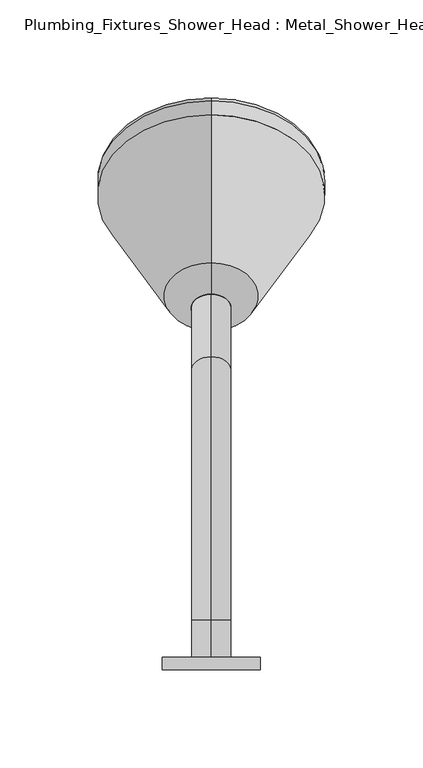
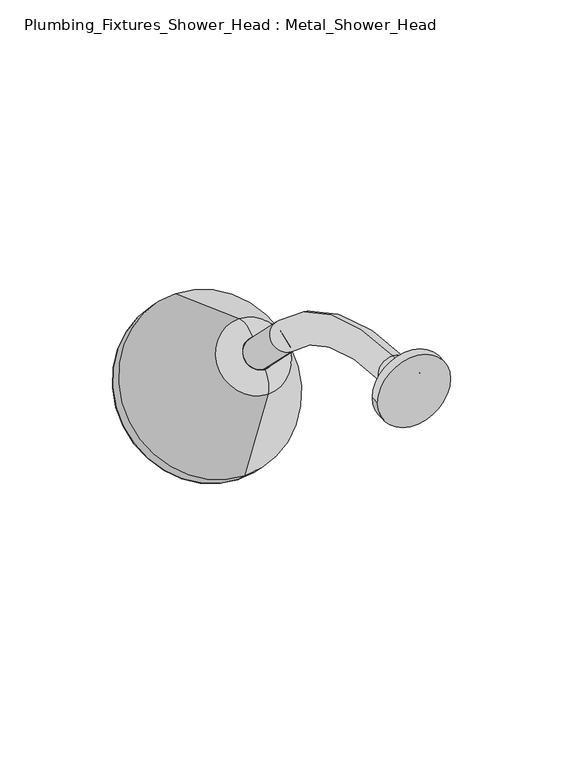
"""IFC4 building model written with IfcOpenShell, lengths in millimetres: flow terminal geometry, Plumbing_Fixtures_Shower_Head : Metal_Shower_Head."""

from ifc_helpers import new_model, si_unit, point, frame, frame_2d, origin, place, context, project, spatial, polyline, circle_curve, ellipse_curve, trimmed, segment, composite_curve, outline, extrude, source, transform, mapped, element, save
from ifc_brep_helpers import plane_surface, cylinder_surface, revolved_surface, advanced_brep


def plumbing_fixtures_shower_head_metal_shower_head_9404fff0(model_context):
    return source(origin(), model_context, "Body", "SolidModel", [
        advanced_brep(
        [(0.0, 6.4821489, 1590.0), (0.0, 6.4821489, 1610.0), (0.0, 25.4415588, 1590.0), (0.0, 25.4415588, 1610.0), (0.0, 159.7918472, 1554.3502884), (0.0, 145.6497116, 1540.2081528), (0.0, 177.4695167, 1508.3883476), (0.0, 191.6116524, 1522.5304833)],
        [
            (0, 1, circle_curve(frame((0.0, 6.4821489, 1600.0), z_axis=(0.0, -1.0, 0.0), x_axis=(0.0, 0.0, 1.0)), 10.0)),
            (1, 0, circle_curve(frame((0.0, 6.4821489, 1600.0), z_axis=(0.0, -1.0, 0.0), x_axis=(0.0, 0.0, 1.0)), 10.0)),
            (0, 2),
            (2, 3, circle_curve(frame((0.0, 25.4415588, 1600.0), z_axis=(0.0, -1.0, 0.0), x_axis=(0.0, 0.0, 1.0)), 10.0)),
            (3, 1),
            (3, 2, circle_curve(frame((0.0, 25.4415588, 1600.0), z_axis=(0.0, -1.0, 0.0), x_axis=(0.0, 0.0, 1.0)), 10.0)),
            (4, 3, circle_curve(frame((0.0, 25.4415588, 1420.0), z_axis=(1.0, 0.0, 0.0), x_axis=(0.0, 0.0, 1.0)), 190.0)),
            (2, 5, circle_curve(frame((0.0, 25.4415588, 1420.0), z_axis=(-1.0, 0.0, 0.0), x_axis=(0.0, 0.0, 1.0)), 170.0)),
            (5, 4, circle_curve(frame((0.0, 152.7207794, 1547.2792206), z_axis=(0.0, -0.7071067811865417, 0.7071067811865533), x_axis=(0.0, 0.7071067811865533, 0.7071067811865417)), 10.0)),
            (4, 5, circle_curve(frame((0.0, 152.7207794, 1547.2792206), z_axis=(0.0, -0.7071067811865416, 0.7071067811865535), x_axis=(0.0, 0.7071067811865535, 0.7071067811865416)), 10.0)),
            (6, 7, circle_curve(frame((0.0, 184.5405845, 1515.4594155), z_axis=(0.0, 0.7071067811865412, -0.7071067811865539), x_axis=(0.0, 0.7071067811865539, 0.7071067811865412)), 10.0)),
            (7, 6, circle_curve(frame((0.0, 184.5405845, 1515.4594155), z_axis=(0.0, 0.7071067811865412, -0.7071067811865539), x_axis=(0.0, 0.7071067811865539, 0.7071067811865412)), 10.0)),
            (5, 6),
            (7, 4),
        ],
        [
            plane_surface(frame((0.0, 6.4821489, 1600.0), z_axis=(0.0, -1.0, 0.0), x_axis=(1.0, 0.0, 0.0))),
            cylinder_surface(frame((0.0, 6.4821489, 1600.0), z_axis=(0.0, -1.0, 0.0), x_axis=(0.0, 0.0, 1.0)), 10.0),
            revolved_surface(trimmed(ellipse_curve(frame((0.0, 25.4415588, 1600.0), z_axis=(0.0, -1.0, 0.0), x_axis=(0.0, 0.0, 1.0)), 10.0, 10.0), [point((0.0, 25.4415588, 1590.0))], [point((0.0, 25.4415588, 1610.0))], True, "CARTESIAN"), (0.0, 25.4415588, 1420.0), (-1.0, 0.0, 0.0)),
            revolved_surface(trimmed(ellipse_curve(frame((0.0, 25.4415588, 1600.0), z_axis=(0.0, -1.0, 0.0), x_axis=(0.0, 0.0, 1.0)), 10.0, 10.0), [point((0.0, 25.4415588, 1610.0))], [point((0.0, 25.4415588, 1590.0))], True, "CARTESIAN"), (0.0, 25.4415588, 1420.0), (-1.0, 0.0, 0.0)),
            plane_surface(frame((0.0, 184.5405845, 1515.4594155), z_axis=(0.0, 0.7071067811865412, -0.7071067811865539), x_axis=(1.0, 0.0, 0.0))),
            cylinder_surface(frame((0.0, 152.7207794, 1547.2792206), z_axis=(0.0, -0.7071067811865412, 0.7071067811865539), x_axis=(0.0, 0.7071067811865539, 0.7071067811865412)), 10.0),
        ],
        [
            (0, [[1, 2]]),
            (1, [[-1, 3, 4, 5]]),
            (1, [[-2, -5, 6, -3]]),
            (2, [[7, -4, 8, 9]]),
            (3, [[-8, -6, -7, 10]]),
            (4, [[11, 12]]),
            (5, [[-9, 13, -12, 14]]),
            (5, [[-10, -14, -11, -13]]),
        ],
    ),
        advanced_brep(
        [(0.0, 207.6624735, 1526.3331882), (0.0, 173.6668118, 1492.3375265), (0.0, 177.1555994, 1508.0744304), (0.0, 191.9255696, 1522.8444006), (0.0, 283.255056, 1498.8197382), (0.0, 201.1802618, 1416.744944), (0.0, 290.3261238, 1491.7486704), (0.0, 208.2513296, 1409.6738762), (0.0, 290.3261238, 1484.6776026), (0.0, 215.3223974, 1409.6738762), (0.0, 288.6229509, 1482.9744296), (0.0, 217.0255704, 1411.3770491), (0.0, 287.2087373, 1484.3886432), (0.0, 215.6113568, 1412.7912627), (0.0, 251.4100471, 1448.5899529), (0.0, 184.5405845, 1515.4594155)],
        [
            (0, 1, circle_curve(frame((0.0, 190.6646427, 1509.3353573), z_axis=(0.0, -0.7071067811865374, 0.7071067811865579), x_axis=(0.0, -0.7071067811865579, -0.7071067811865374)), 24.0385629)),
            (1, 2, circle_curve(frame((0.0, 187.7622012, 1497.4678286), z_axis=(-1.0000000000000002, 0.0, 0.0), x_axis=(0.0, 1.0000000000000002, 0.0)), 15.0)),
            (2, 3, circle_curve(frame((0.0, 184.5405845, 1515.4594155), z_axis=(0.0, 0.7071067811865374, -0.7071067811865579), x_axis=(0.0, -0.7071067811865579, -0.7071067811865374)), 10.4439461)),
            (3, 0, circle_curve(frame((0.0, 202.5321714, 1512.2377988), z_axis=(-1.0000000000000002, 0.0, 0.0), x_axis=(0.0, 0.0, -1.0000000000000002)), 15.0)),
            (1, 0, circle_curve(frame((0.0, 190.6646427, 1509.3353573), z_axis=(0.0, -0.7071067811865374, 0.7071067811865579), x_axis=(0.0, -0.7071067811865579, -0.7071067811865374)), 24.0385629)),
            (3, 2, circle_curve(frame((0.0, 184.5405845, 1515.4594155), z_axis=(0.0, 0.7071067811865374, -0.7071067811865579), x_axis=(0.0, -0.7071067811865579, -0.7071067811865374)), 10.4439461)),
            (4, 5, circle_curve(frame((0.0, 242.2176589, 1457.7823411), z_axis=(0.0, -0.7071067811865374, 0.7071067811865579), x_axis=(0.0, -0.7071067811865579, -0.7071067811865374)), 58.0356436)),
            (5, 1),
            (0, 4),
            (5, 4, circle_curve(frame((0.0, 242.2176589, 1457.7823411), z_axis=(0.0, -0.7071067811865374, 0.7071067811865579), x_axis=(0.0, -0.7071067811865579, -0.7071067811865374)), 58.0356436)),
            (6, 7, circle_curve(frame((0.0, 249.2887267, 1450.7112733), z_axis=(0.0, -0.7071067811865374, 0.7071067811865579), x_axis=(0.0, -0.7071067811865579, -0.7071067811865374)), 58.0356436)),
            (7, 5),
            (4, 6),
            (7, 6, circle_curve(frame((0.0, 249.2887267, 1450.7112733), z_axis=(0.0, -0.7071067811865374, 0.7071067811865579), x_axis=(0.0, -0.7071067811865579, -0.7071067811865374)), 58.0356436)),
            (8, 9, circle_curve(frame((0.0, 252.8242606, 1447.1757394), z_axis=(0.0, -0.7071067811865374, 0.7071067811865579), x_axis=(0.0, -0.7071067811865579, -0.7071067811865374)), 53.0356436)),
            (9, 7, circle_curve(frame((0.0, 211.7868635, 1413.2094101), z_axis=(-1.0000000000000002, 0.0, 0.0), x_axis=(0.0, 1.0000000000000002, 0.0)), 5.0)),
            (6, 8, circle_curve(frame((0.0, 286.7905899, 1488.2131365), z_axis=(-1.0000000000000002, 0.0, 0.0), x_axis=(0.0, 0.0, -1.0000000000000002)), 5.0)),
            (9, 8, circle_curve(frame((0.0, 252.8242606, 1447.1757394), z_axis=(0.0, -0.7071067811865374, 0.7071067811865579), x_axis=(0.0, -0.7071067811865579, -0.7071067811865374)), 53.0356436)),
            (10, 11, circle_curve(frame((0.0, 252.8242606, 1447.1757394), z_axis=(0.0, -0.7071067811865374, 0.7071067811865579), x_axis=(0.0, -0.7071067811865579, -0.7071067811865374)), 50.6269933)),
            (11, 9),
            (8, 10),
            (11, 10, circle_curve(frame((0.0, 252.8242606, 1447.1757394), z_axis=(0.0, -0.7071067811865374, 0.7071067811865579), x_axis=(0.0, -0.7071067811865579, -0.7071067811865374)), 50.6269933)),
            (12, 13, circle_curve(frame((0.0, 251.4100471, 1448.5899529), z_axis=(0.0, -0.7071067811865374, 0.7071067811865579), x_axis=(0.0, -0.7071067811865579, -0.7071067811865374)), 50.6269933)),
            (13, 11),
            (10, 12),
            (13, 12, circle_curve(frame((0.0, 251.4100471, 1448.5899529), z_axis=(0.0, -0.7071067811865374, 0.7071067811865579), x_axis=(0.0, -0.7071067811865579, -0.7071067811865374)), 50.6269933)),
            (14, 13),
            (12, 14),
            (2, 15),
            (15, 3),
        ],
        [
            revolved_surface(trimmed(ellipse_curve(frame((0.0, 187.7622012, 1497.4678286), z_axis=(1.0000000000000002, 0.0, 0.0), x_axis=(0.0, 1.0000000000000002, 0.0)), 15.0, 15.0), [point((0.0, 177.1555994, 1508.0744304))], [point((0.0, 173.6668118, 1492.3375265))], True, "CARTESIAN"), (0.0, 184.5405845, 1515.4594155), (0.0, 0.7071067811865374, -0.7071067811865579)),
            revolved_surface(polyline([(0.0, 173.6668118, 1492.3375265), (0.0, 201.1802618, 1416.744944)]), (0.0, 184.5405845, 1515.4594155), (0.0, 0.7071067811865374, -0.7071067811865579)),
            cylinder_surface(frame((0.0, 184.5405845, 1515.4594155), z_axis=(0.0, 0.7071067811865374, -0.7071067811865579), x_axis=(0.0, -0.7071067811865579, -0.7071067811865374)), 58.0356436),
            revolved_surface(trimmed(ellipse_curve(frame((0.0, 211.7868635, 1413.2094101), z_axis=(1.0000000000000002, 0.0, 0.0), x_axis=(0.0, 1.0000000000000002, 0.0)), 5.0, 5.0), [point((0.0, 208.2513296, 1409.6738762))], [point((0.0, 215.3223974, 1409.6738762))], True, "CARTESIAN"), (0.0, 184.5405845, 1515.4594155), (0.0, 0.7071067811865374, -0.7071067811865579)),
            plane_surface(frame((0.0, 252.8242606, 1447.1757394), z_axis=(0.0, 0.7071067811865374, -0.7071067811865579), x_axis=(0.0, -0.7071067811865579, -0.7071067811865374))),
            revolved_surface(polyline([(0.0, 217.02557037648307, 1411.3770490764832), (0.0, 215.61135677648213, 1412.7912626764842)]), (0.0, 184.5405845, 1515.4594155), (0.0, 0.7071067811865374, -0.7071067811865579)),
            plane_surface(frame((0.0, 251.4100471, 1448.5899529), z_axis=(0.0, 0.7071067811865374, -0.7071067811865579), x_axis=(0.0, -0.7071067811865579, -0.7071067811865374))),
            plane_surface(frame((0.0, 184.5405845, 1515.4594155), z_axis=(0.0, -0.7071067811865374, 0.7071067811865579), x_axis=(0.0, -0.7071067811865579, -0.7071067811865374))),
        ],
        [
            (0, [[1, 2, 3, 4]]),
            (0, [[5, -4, 6, -2]]),
            (1, [[7, 8, -1, 9]]),
            (1, [[10, -9, -5, -8]]),
            (2, [[11, 12, -7, 13]]),
            (2, [[14, -13, -10, -12]]),
            (3, [[15, 16, -11, 17]]),
            (3, [[18, -17, -14, -16]]),
            (4, [[19, 20, -15, 21]]),
            (4, [[22, -21, -18, -20]]),
            (5, [[23, 24, -19, 25]]),
            (5, [[26, -25, -22, -24]]),
            (6, [[27, -23, 28]]),
            (6, [[-28, -26, -27]]),
            (7, [[-3, 29, 30]]),
            (7, [[-6, -30, -29]]),
        ],
    ),
        extrude(outline(composite_curve([segment(trimmed(circle_curve(frame_2d((1600.0, 0.0)), 25.0), [point((1600.0, -25.0))], [point((1600.0, 25.0))], False, "CARTESIAN"), True, "CONTINUOUS"), segment(trimmed(circle_curve(frame_2d((1600.0, 0.0)), 25.0), [point((1600.0, 25.0))], [point((1600.0, -25.0))], False, "CARTESIAN"), True, "CONTINUOUS")], self_intersect=False)), frame((0.0, 0.0, 0.0), z_axis=(0.0, 1.0, 0.0), x_axis=(0.0, 0.0, 1.0)), (0.0, 0.0, 1.0), 6.4821489),
    ])


if __name__ == "__main__":
    model = new_model("IFC4")
    model_context = context("Model", 3, world=origin())
    ifc_project = project(units=[si_unit("LENGTHUNIT", "METRE", prefix="MILLI")], contexts=[model_context])
    site = spatial("IfcSite", under=ifc_project)
    building = spatial("IfcBuilding", under=site)
    placement = place(None, origin())
    plumbing_fixtures_shower_head_metal_shower_head_shape = plumbing_fixtures_shower_head_metal_shower_head_9404fff0(model_context)
    element("IfcFlowTerminal", 1, ObjectType="Plumbing_Fixtures_Shower_Head : Metal_Shower_Head", at=placement, inside=building, context=model_context, shape_type="MappedRepresentation", body=[
        mapped(plumbing_fixtures_shower_head_metal_shower_head_shape, transform((0.0, 0.0, 0.0), x_axis=(1.0, 0.0, 0.0), y_axis=(0.0, 1.0, 0.0), z_axis=(0.0, 0.0, 1.0))),
    ])
    save(model, "model.ifc")

# Revit data of these elements
# Type "Plumbing_Fixtures_Shower_Head : Metal_Shower_Head"
#   Keynote = "N13/230"
#   Mounting Height = 5.249344 ft
#   Material Shower Head = Metal - Chrome Polished
#   Default Elevation = 0
# Element 1 (IfcFlowTerminal, "Plumbing_Fixtures_Shower_Head : Metal_Shower_Head")
#   Materials on its faces: "Metal - Chrome Polished"
# Materials
#   "Metal - Chrome Polished": colour RGB 247 247 247, transparency 0
